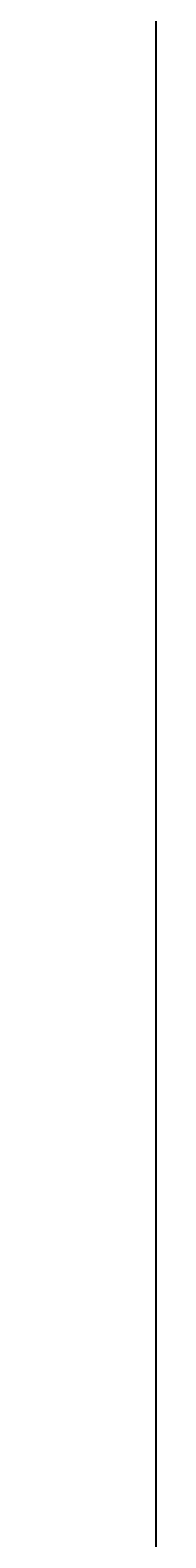
# Model space of a CAD drawing. Units: inches. Extents: x 1998 to 2588, y 1139 to 1977.
# Tile 56 of 134: x 2220 to 2223, y 1708 to 1746. Entities that reach past the tile are written whole.
import ezdxf

# ---------------------------------------------------------------- set-up
doc = ezdxf.new("R2010")
doc.units = ezdxf.units.IN
doc.layers.add('A-ANNO-DIMS', color=2, linetype='Continuous', lineweight=18)
doc.styles.get("Standard").update_dxf_attribs({"font": 'arial.ttf'})
doc.dimstyles.get("Standard").update_dxf_attribs({"dimtxt": 0.18, "dimasz": 0.18, "dimexe": 0.18, "dimexo": 0.0625, "dimgap": 0.09, "dimtad": 0, "dimtih": 1, "dimtoh": 1, "dimdec": 4, "dimzin": 0, "dimdsep": 46, "dimtxsty": 'Standard', "dimcen": 0.09, "dimadec": 0, "dimazin": 0, "dimtfac": 1, "dimtdec": 4, "dimtofl": 0, "dimtmove": 0, "dimatfit": 3, "dimfxl": 1, "dimtolj": 1, "dimtzin": 0, "dimarcsym": 0})

# ---------------------------------------------------------------- blocks, each defined once
blk = doc.blocks.new('*D36')
at = {"layer": 'A-ANNO-DIMS', "color": 0, "lineweight": -2, "transparency": 16777216}
for p, q in [((2197.45, 1663.309), (2197.45, 1977.362)), ((2197.63, 1977.182), (2209.746, 1977.182)), ((2222.793, 1977.182), (2210.677, 1977.182)), ((2222.973, 1663.309), (2222.973, 1977.362))]:
    blk.add_line(p, q, dxfattribs=at)
at = {"layer": 'A-ANNO-DIMS', "color": 0, "transparency": 16777216}
for points in [[(2197.63, 1977.212), (2197.63, 1977.152), (2197.45, 1977.182)], [(2222.793, 1977.212), (2222.793, 1977.152), (2222.973, 1977.182)]]:
    blk.add_solid(points, dxfattribs=at)
at = {"layer": 'Defpoints', "color": 0, "transparency": 16777216}
for p in [(2222.973, 1977.182), (2197.45, 1663.247), (2222.973, 1663.247)]:
    blk.add_point(p, dxfattribs=at)
at = {"layer": 'A-ANNO-DIMS', "color": 0, "transparency": 16777216, "insert": (2210.211, 1977.182), "char_height": 0.18, "attachment_point": 5}
blk.add_mtext('\\A1;25.523', dxfattribs=at)

msp = doc.modelspace()

# ---------------------------------------------------------------- dimensions: what is measured, and where the dimension line sits
at = {"layer": 'A-ANNO-DIMS'}
dim = msp.add_linear_dim(base=(2222.9729, 1977.1824), p1=(2197.4499, 1663.2466), p2=(2222.9729, 1663.2466), dimstyle='Standard', override={"dimdec": 3, "dimlfac": 1, "dimrnd": 0, "dimzin": 0, "dimdsep": 46, "dimlunit": 2}, dxfattribs=at)
dim.commit()
dim.dimension.update_dxf_attribs({"geometry": '*D36', "text_midpoint": (2210.2114, 1977.1824)})

doc.saveas('drawing.dxf')
